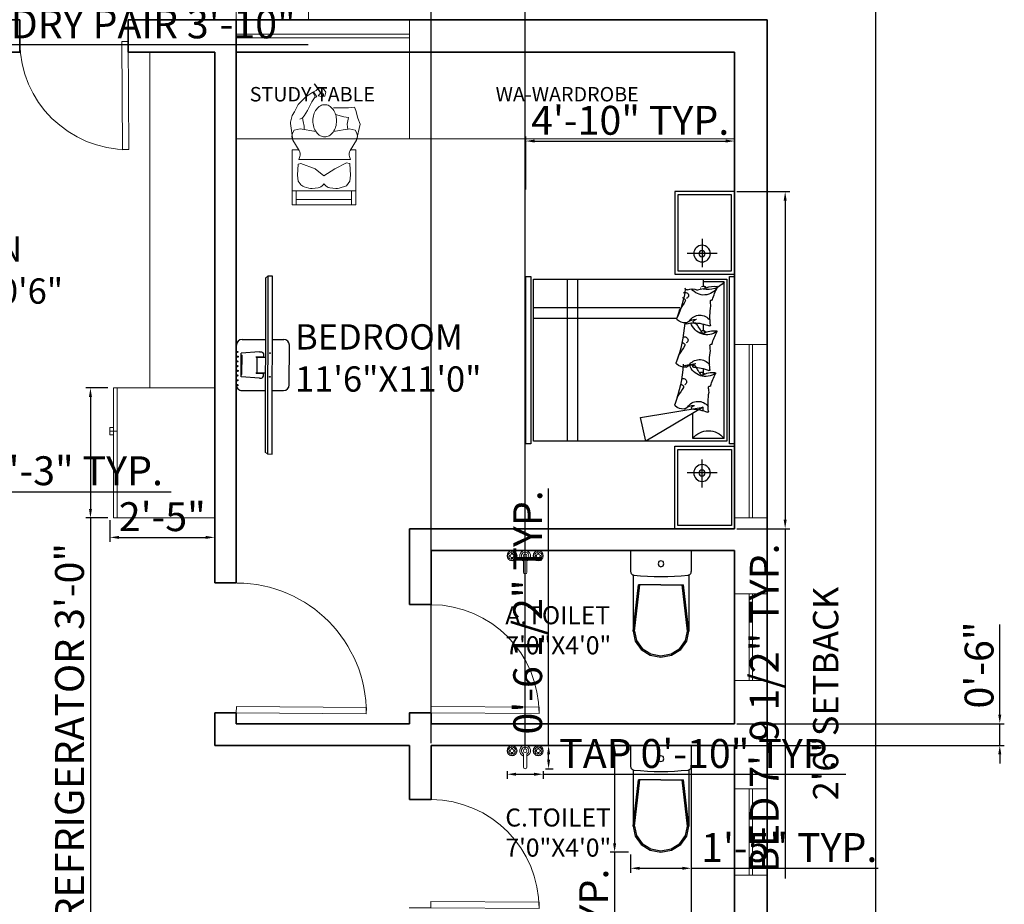
# Model space of a CAD drawing. Units: inches. Extents: x 3394 to 4794, y 965 to 1718.
# Tile 10 of 15: x 3704 to 3976, y 1338 to 1583. Entities that reach past the tile are written whole.
import ezdxf

# ---------------------------------------------------------------- set-up
doc = ezdxf.new("R2010")
doc.units = ezdxf.units.IN
for name, color, linetype, lineweight in [('A-ANNO-DIMS', 2, 'Continuous', 13), ('A-ANNO-TEXT', 7, 'Continuous', 18), ('A-AREA-IDEN', 7, 'Continuous', 18), ('A-DOOR', 4, 'Continuous', 18), ('A-EQPM', 8, 'Continuous', 18), ('A-FLOR-CASE', 8, 'Continuous', 18), ('A-FLOR-STRS', 7, 'Continuous', 18), ('A-GLAZ', 4, 'Continuous', 18), ('A-WALL', 7, 'Continuous', 35), ('C-PROP', 7, 'Continuous', 25), ('NOITHAT', 21, 'Continuous', 18), ('Сантехника', 7, 'Continuous', 18)]:
    doc.layers.add(name, color=color, linetype=linetype, lineweight=lineweight)
for name, color, linetype in [('FUR', 42, 'Continuous'), ('HA', 9, 'Continuous'), ('HID', 11, 'Continuous'), ('SAN', 5, 'Continuous'), ('SANTEH', 7, 'Continuous'), ('window', 130, 'Continuous')]:
    doc.layers.add(name, color=color, linetype=linetype)
doc.styles.get("Standard").update_dxf_attribs({"font": 'arial.ttf'})
doc.dimstyles.new('ISO-25', dxfattribs={"dimtxt": 8, "dimasz": 2.5, "dimexe": 1.25, "dimexo": 0.625, "dimtad": 1, "dimlunit": 3, "dimtxsty": 'Standard', "dimcen": 2.5, "dimadec": 0, "dimazin": 0, "dimtfac": 1, "dimtmove": 0, "dimatfit": 3, "dimfxl": 1, "dimarcsym": 0})

# ---------------------------------------------------------------- blocks, each defined once
blk = doc.blocks.new('Refrigerator-2 door - 36 in top')
for p, q in [((0, -26.999999), (36, -26.999999)), ((12, -26.999999), (12, -28.999999)), ((11, -27.999999), (11, -28.999999)), ((11, -28.999999), (13, -28.999999)), ((13, -28.999999), (13, -27.999999))]:
    blk.add_line(p, q)
blk.add_lwpolyline([(0, -27.999999), (0, 0), (36, 0), (36, -27.999999)], close=True)
blk = doc.blocks.new('Faucet - Bathroom top')
for p, q in [((-4.107, 0.125), (-4.375, 0.125)), ((-3.75, 0.4788), (-3.75, 0.75)), ((-3.5, 0.482), (-3.5, 0.75)), ((-3.1461, 0.125), (-2.875, 0.125)), ((3.143, 0.125), (2.875, 0.125)), ((3.5, 0.4788), (3.5, 0.75)), ((3.75, 0.482), (3.75, 0.75)), ((4.1039, 0.125), (4.375, 0.125)), ((-4.1039, -0.125), (-4.375, -0.125)), ((-3.75, -0.4821), (-3.75, -0.75)), ((-3.5, -0.4789), (-3.5, -0.75)), ((-3.143, -0.125), (-2.875, -0.125)), ((-0.5, -0.8639), (-0.5, -4.5)), ((0.5, -4.5), (0.5, -0.8631)), ((3.1461, -0.125), (2.875, -0.125)), ((3.5, -0.4821), (3.5, -0.75)), ((3.75, -0.4789), (3.75, -0.75)), ((4.107, -0.125), (4.375, -0.125))]:
    blk.add_line(p, q)
for centre, radius in [((-3.625, 0), 1.375), ((-4.625, 0), 0.2795), ((-3.625, 0), 0.5), ((-3.625, 1), 0.2795), ((-2.625, 0), 0.2795), ((0, 0), 0.5), ((3.625, 0), 1.375), ((2.625, 0), 0.2795), ((3.625, 0), 0.5), ((3.625, 1), 0.2795), ((4.625, 0), 0.2795), ((-3.625, -1), 0.2795), ((3.625, -1), 0.2795)]:
    blk.add_circle(centre, radius)
for centre, radius, start, end in [((-3.625, 0), 1, 105.2407, 164.2093), ((-3.625, 0), 1, 16.44125, 74.07887), ((0, 0), 1.5, 289.6514, 250.3603), ((0, 0), 1, 300.3431, 239.7554), ((3.625, 0), 1, 106.12, 164.0884), ((3.625, 0), 1, 16.23422, 73.90469), ((-3.625, 0), 1, 196.2342, 253.9047), ((-3.625, 0), 1, 286.12, 344.0884), ((3.625, 0), 1, 196.4413, 254.0789), ((3.625, 0), 1, 285.2407, 344.2093), ((0, -4.5), 0.5, 180, 0)]:
    blk.add_arc(centre, radius, start, end)
blk = doc.blocks.new('*U5')
for p, q in [((0, 0), (0, -6)), ((30, 0), (30, -6))]:
    blk.add_line(p, q)
blk.add_lwpolyline([(0, 0), (0, 30), (1.75, 30), (1.75, 0)], close=True)
blk.add_arc((0, 0), 30, 0, 90)
blk = doc.blocks.new('WC 2 Symb_109')
at = {"layer": 'SANTEH'}
for p, q in [((0, 0), (0, 380)), ((0, 380), (132.4, 380)), ((153.6, 364.9), (506.8, 364.9)), ((506.3, 364.9), (215.7, 330.9)), ((506.3, 356), (215.7, 322)), ((215.7, 190), (215.7, 330.9)), ((215.7, 190), (215.7, 49.1)), ((153.8, 15.1), (506.8, 15.1)), ((506.3, 24), (215.7, 58)), ((506.3, 15.1), (215.7, 49.1)), ((0, 0), (132.4, 0))]:
    blk.add_line(p, q, dxfattribs=at)
for points in [[(154.6, 360.1), (153.9, 364.1), (152.3, 367.9), (150.2, 371.3), (147.4, 374.3), (144.1, 376.7), (140.5, 378.5), (136.5, 379.6), (132.4, 380)], [(154.6, 19.7), (158.6, 62.1), (161.4, 104.7), (163.1, 147.3), (163.7, 189.9), (163.1, 232.5), (161.4, 275.1), (158.6, 317.7), (154.6, 360.1)], [(506.3, 24), (565.5, 36.6), (615.7, 72.6), (649.2, 126.5), (661, 190), (649.2, 253.5), (615.7, 307.4), (565.5, 343.4), (506.3, 356)], [(506.8, 15.1), (569.2, 28.4), (622.2, 66.3), (657.6, 123.1), (670, 190), (657.6, 256.9), (622.2, 313.7), (569.2, 351.6), (506.8, 364.9)], [(132.4, 0), (136.5, 0.4), (140.4, 1.5), (144.1, 3.2), (147.3, 5.6), (150.1, 8.6), (152.3, 12), (153.8, 15.7), (154.6, 19.7)]]:
    blk.add_lwpolyline(points, dxfattribs=at)
blk.add_lwpolyline([(83.6, 208.5), (70.4, 203.1), (64.9, 190), (70.4, 176.9), (83.6, 171.5), (96.8, 176.9), (102.2, 190), (96.8, 203.1)], close=True, dxfattribs=at)
blk = doc.blocks.new('*U11')
for p, q in [((0, 0), (0, -6)), ((36, 0), (36, -6))]:
    blk.add_line(p, q)
blk.add_lwpolyline([(0, 0), (0, 36), (1.75, 36), (1.75, 0)], close=True)
blk.add_arc((0, 0), 36, 0, 90)
blk = doc.blocks.new('A$C73A16738')
at = {"layer": 'FUR'}
for p, q in [((1.15, 2.3893), (1.1, 2.1643)), ((1.7, 2.0643), (1.15, 2.3893)), ((1.6, 2.3643), (1.6, 2.1234)), ((1.9, 2.3643), (1.6, 2.3643)), ((1.9, 2.3643), (1.9, 0.8643)), ((1.1, 2.1643), (1.7, 2.0643)), ((1.7, 2.099), (1.7, 2.0643)), ((1.7, 1.6955), (1.7, 1.7349)), ((1.7, 1.2682), (1.7, 1.3299)), ((1.7, 0.8393), (1.7, 0.9036)), ((1.9, 0.8643), (1.7, 0.8643))]:
    blk.add_line(p, q, dxfattribs=at)
for points in [[(1.428, 2.4393), (2, 2.4393), (2, 3.2287), (1.428, 3.2287)], [(1.458, 2.4693), (1.97, 2.4693), (1.97, 3.1987), (1.458, 3.1987)], [(0, 2.4143), (0, 0.8143), (0.05, 0.8143), (0.05, 2.4143)], [(0.075, 0.8393), (1.925, 0.8393), (1.925, 2.3893), (0.075, 2.3893)], [(1.95, 2.4143), (1.95, 0.8143), (2, 0.8143), (2, 2.4143)], [(1.428, 0.7893), (2, 0.7893), (2, 0), (1.428, 0)], [(1.458, 0.7593), (1.97, 0.7593), (1.97, 0.03), (1.458, 0.03)]]:
    blk.add_lwpolyline(points, close=True, dxfattribs=at)
for centre, start, end in [((1.75, 2.4806), 217.78263, 322.21737), ((1.75, 0.7481), 37.78263, 105.27469)]:
    blk.add_arc(centre, 0.1898, start, end, dxfattribs=at)
at = {"layer": 'HA'}
for p, q in [((0.4, 2.3893), (0.4, 0.8393)), ((0.5, 2.3893), (0.5, 0.8393)), ((1.4456, 1.2143), (0.075, 1.2143)), ((1.4772, 1.1143), (0.075, 1.1143))]:
    blk.add_line(p, q, dxfattribs=at)
at = {"layer": 'HID'}
for centre, radius, start, end in [((1.5102, 1.9654), 0.1174, 87.33771, 131.66603), ((1.515, 2.0683), 0.0144, 51.60711, 87.33771), ((1.6169, 2.1969), 0.1496, 231.60711, 269.78448), ((1.5925, 2.0742), 0.0072, 92.73629, 208.29854), ((1.5692, 2.5605), 0.4796, 272.73629, 290.95899), ((1.7434, 2.1059), 0.0072, 352.72477, 110.95899), ((2.3483, 2.0286), 0.6026, 172.72477, 190.27016), ((1.4417, 2.0424), 0.0144, 131.66603, 199.44651), ((0.016, 1.539), 1.4976, 4.58522, 19.44651), ((0.016, 1.539), 1.4976, 16.38601, 19.44651), ((1.6496, 2.1284), 0.1197, 212.76276, 323.89219), ((1.628, 2.0933), 0.0475, 208.29854, 255.78909), ((1.4666, 1.9655), 0.0144, 196.38601, 223.79553), ((0.9264, 1.5508), 0.6667, 29.04896, 37.38232), ((2.0379, 1.8684), 0.2875, 169.41677, 179.30852), ((1.5097, 1.8233), 0.0319, 112.70152, 147.15561), ((1.5097, 1.8214), 0.0305, 232.35651, 65.77621), ((1.5029, 1.8394), 0.0144, 102.64257, 112.70152), ((1.4966, 1.8675), 0.0144, 282.64257, 29.04896), ((1.7576, 1.8718), 0.0072, 179.30852, 290.68903), ((1.7627, 1.8583), 0.0072, 16.21957, 110.68903), ((2.3483, 2.0286), 0.6026, 196.21957, 208.21138), ((1.7225, 1.6087), 0.1623, 53.89466, 162.39517), ((1.5829, 2.1606), 0.4796, 272.73629, 290.95899), ((2.8537, 0.9606), 1.4182, 145.83293, 150.02451), ((3.1426, 2.3695), 1.6108, 202.70178, 202.72062), ((1.6834, 1.7584), 0.0288, 232.66199, 339.15728), ((1.6862, 1.7531), 0.0072, 38.83153, 145.83293), ((1.788, 1.9236), 0.1919, 239.92106, 277.12402), ((0.088, 1.8308), 1.6108, 356.49824, 357.28883), ((1.7571, 1.706), 0.0072, 352.72477, 110.95899), ((2.362, 1.6287), 0.6026, 172.72477, 190.27016), ((1.8109, 1.7404), 0.0072, 277.12402, 28.21138), ((1.8109, 1.7404), 0.0072, 277.12402, 28.21138), ((1.4554, 1.6425), 0.0144, 131.66603, 199.44651), ((0.0297, 1.1391), 1.4976, 4.58522, 19.44651), ((0.0297, 1.1391), 1.4976, 16.38601, 19.44651), ((1.5239, 1.5655), 0.1174, 87.33771, 131.66603), ((1.5236, 1.6535), 0.0144, 67.16626, 184.34216), ((1.5745, 1.7743), 0.1167, 247.16626, 295.7613), ((1.5287, 1.6684), 0.0144, 51.60711, 87.33771), ((1.6306, 1.797), 0.1496, 231.60711, 269.78448), ((1.6633, 1.7284), 0.1197, 212.76276, 323.89219), ((1.6062, 1.6743), 0.0072, 92.73629, 208.29854), ((1.6417, 1.6934), 0.0475, 208.29854, 255.78909), ((1.4803, 1.5656), 0.0144, 196.38601, 223.79553), ((0.9401, 1.1509), 0.6667, 29.04896, 37.38232), ((2.0516, 1.4685), 0.2875, 169.41677, 179.30852), ((1.5234, 1.4234), 0.0319, 112.70152, 147.15561), ((1.5234, 1.4215), 0.0305, 232.35651, 65.77621), ((1.5166, 1.4395), 0.0144, 102.64257, 112.70152), ((1.5103, 1.4676), 0.0144, 282.64257, 29.04896), ((1.7713, 1.4719), 0.0072, 179.30852, 290.68903), ((1.7764, 1.4584), 0.0072, 16.21957, 110.68903), ((2.362, 1.6287), 0.6026, 196.21957, 208.21138), ((1.7362, 1.2088), 0.1623, 53.89466, 162.39517), ((2.8674, 0.5607), 1.4182, 145.83293, 150.02451), ((3.1563, 1.9695), 1.6108, 202.70178, 202.72062), ((1.6971, 1.3585), 0.0288, 232.66199, 339.15728), ((1.6999, 1.3531), 0.0072, 38.83153, 145.83293), ((1.8017, 1.5237), 0.1919, 239.92106, 277.12402), ((0.1017, 1.4309), 1.6108, 356.49824, 357.28883), ((1.8246, 1.3404), 0.0072, 277.12402, 28.21138), ((1.8246, 1.3404), 0.0072, 277.12402, 28.21138), ((1.4601, 1.2163), 0.0144, 131.66603, 199.44651), ((1.5286, 1.1394), 0.1174, 87.33771, 131.66603), ((1.5373, 1.2536), 0.0144, 67.16626, 184.34216), ((1.5334, 1.2423), 0.0144, 51.60711, 87.33771), ((1.6353, 1.3709), 0.1496, 231.60711, 269.78448), ((1.5882, 1.3744), 0.1167, 247.16626, 295.7613), ((1.6681, 1.3023), 0.1197, 212.76276, 323.89219), ((1.6109, 1.2482), 0.0072, 92.73629, 208.29854), ((1.6464, 1.2673), 0.0475, 208.29854, 255.78909), ((1.5877, 1.7344), 0.4796, 272.73629, 290.95899), ((1.7618, 1.2798), 0.0072, 352.72477, 110.95899), ((2.3667, 1.2026), 0.6026, 172.72477, 190.27016), ((0.6883, 0.8412), 0.8439, 6.22401, 26.03262), ((0.0344, 0.713), 1.4976, 16.38601, 19.44651), ((1.485, 1.1395), 0.0144, 196.38601, 223.79553), ((0.9449, 0.7248), 0.6667, 29.04896, 37.38232), ((1.5151, 1.0415), 0.0144, 282.64257, 29.04896), ((2.0564, 1.0424), 0.2875, 169.41677, 179.30852), ((1.7761, 1.0457), 0.0072, 179.30852, 290.68903), ((1.7812, 1.0323), 0.0072, 16.21957, 110.68903), ((1.5281, 0.9972), 0.0319, 112.70152, 147.15561), ((1.5282, 0.9954), 0.0305, 232.35651, 65.77621), ((1.5214, 1.0134), 0.0144, 102.64257, 112.70152), ((1.5929, 1.0482), 0.1167, 247.16626, 295.7613), ((1.7054, 0.84), 0.1504, 29.35981, 142.42811), ((1.5813, 0.5283), 0.4195, 73.75237, 81.4605), ((2.3667, 1.2026), 0.6026, 196.21957, 208.21138), ((1.5421, 0.9274), 0.0144, 67.16626, 184.34216), ((3.1611, 1.5434), 1.6108, 202.70178, 202.72062), ((1.7018, 0.9324), 0.0288, 232.66199, 339.15728), ((1.7047, 0.927), 0.0072, 38.83153, 145.83293), ((0.1065, 1.0048), 1.6108, 356.49824, 357.28883), ((1.8064, 1.0976), 0.1919, 246.10926, 277.12402), ((1.8293, 0.9143), 0.0072, 277.12402, 28.21138), ((1.8293, 0.9143), 0.0072, 277.12402, 28.21138)]:
    blk.add_arc(centre, radius, start, end, dxfattribs=at)
at = {"layer": 'SAN'}
for p, q in [((1.6885, 2.8351), (1.6885, 2.5658)), ((1.8316, 2.6947), (1.5465, 2.6947)), ((1.6885, 0.4536), (1.6885, 0.7229)), ((1.8316, 0.594), (1.5465, 0.594))]:
    blk.add_line(p, q, dxfattribs=at)
for centre, radius in [((1.6885, 2.6947), 0.08), ((1.6885, 2.6947), 0.03), ((1.6885, 0.594), 0.08), ((1.6885, 0.594), 0.03)]:
    blk.add_circle(centre, radius, dxfattribs=at)
blk = doc.blocks.new('TV')
at = {"color": 0}
for p, q in [((3967.27, 1784.85), (3967.05, 1784.65)), ((3967.76, 1763.68), (3967.54, 1763.86))]:
    blk.add_line(p, q, dxfattribs=at)
at = {"layer": 'window'}
for p, q in [((3967.54, 1763.86), (3967.05, 1784.65)), ((3964.41, 1777.23), (3967.22, 1777.3)), ((3968.01, 1777.32), (3969.36, 1777.35)), ((3966.53, 1775.82), (3964.33, 1775.61)), ((3964.34, 1775.34), (3964.45, 1775.34)), ((3964.34, 1775.31), (3964.43, 1775.32)), ((3966.14, 1775.2), (3967.01, 1775.22)), ((3966.14, 1775.18), (3967.27, 1775.2)), ((3966.14, 1775.18), (3966.14, 1775.2)), ((3966.3, 1773.29), (3966.26, 1775.18)), ((3964.39, 1773.06), (3964.48, 1773.06)), ((3964.39, 1773.04), (3964.5, 1773.04)), ((3966.19, 1773.28), (3967.31, 1773.31)), ((3966.19, 1773.26), (3967.05, 1773.28)), ((3966.19, 1773.26), (3966.19, 1773.28)), ((3966.61, 1772.66), (3964.4, 1772.77)), ((3964.55, 1771.15), (3967.36, 1771.22)), ((3968.15, 1771.24), (3969.5, 1771.27))]:
    blk.add_line(p, q, dxfattribs=at)
for points in [[(3968.33, 1763.69), (3967.83, 1784.86), (3967.27, 1784.85), (3967.76, 1763.68), (3968.33, 1763.69)], [(3963.86, 1771.81), (3963.75, 1776.54)], [(3970.16, 1771.96), (3970.05, 1776.69)], [(3964.4, 1772.77), (3964.33, 1775.61)], [(3964.48, 1773.06), (3964.43, 1775.32)], [(3964.5, 1773.04), (3964.45, 1775.34)]]:
    blk.add_lwpolyline(points, dxfattribs=at)
for points in [[(3966.53, 1775.82, -0.263666), (3966.93, 1775.69), (3967, 1775.57), (3967.01, 1775.22)], [(3966.61, 1772.66, 0.263666), (3967, 1772.81), (3967.06, 1772.93), (3967.05, 1773.28)]]:
    blk.add_lwpolyline(points, format="xyb", dxfattribs=at)
for centre, radius in [((3963.91, 1775.73), 0.0679), ((3963.93, 1775.17), 0.0679), ((3967.77, 1775.68), 0.0451), ((3963.94, 1774.6), 0.0679), ((3963.95, 1774.04), 0.0679), ((3963.97, 1773.48), 0.0679), ((3963.98, 1772.92), 0.0679), ((3967.83, 1772.86), 0.0451), ((3963.99, 1772.35), 0.0679), ((3964.01, 1771.79), 0.0679)]:
    blk.add_circle(centre, radius, dxfattribs=at)
for centre, start, end in [((3964.42, 1776.56), 91.3414, 181.3414), ((3969.38, 1776.67), 1.3414, 91.3414), ((3964.53, 1771.83), 181.3414, 271.3414), ((3969.49, 1771.94), 271.3414, 1.3414)]:
    blk.add_arc(centre, 0.676, start, end, dxfattribs=at)
blk = doc.blocks.new('WIN-48IN')
for p, q in [((9, 48), (0, 48)), ((4, 0), (4, 48)), ((5, 0), (5, 48)), ((9, 0), (0, 0))]:
    blk.add_line(p, q)
blk = doc.blocks.new('WIN-24IN')
for p, q in [((0, 9), (0, 0)), ((24, 9), (24, 0)), ((0, 5), (24, 5)), ((0, 4), (24, 4))]:
    blk.add_line(p, q)
blk = doc.blocks.new('*D78')
at = {"layer": 'A-ANNO-DIMS', "color": 0, "lineweight": -2, "transparency": 16777216}
for p, q in [((3838.73, 1374.56), (3838.73, 1372.43)), ((3848.73, 1374.56), (3848.73, 1372.43)), ((3841.23, 1373.68), (3846.23, 1373.68)), ((3848.73, 1373.68), (3932.51, 1373.68))]:
    blk.add_line(p, q, dxfattribs=at)
at = {"layer": 'A-ANNO-DIMS', "color": 0, "transparency": 16777216}
for points in [[(3841.23, 1374.1), (3841.23, 1373.27), (3838.73, 1373.68)], [(3846.23, 1374.1), (3846.23, 1373.27), (3848.73, 1373.68)]]:
    blk.add_solid(points, dxfattribs=at)
at = {"layer": 'Defpoints', "color": 0, "transparency": 16777216}
for p in [(3838.73, 1375.18), (3848.73, 1375.18), (3848.73, 1373.68)]:
    blk.add_point(p, dxfattribs=at)
at = {"layer": 'A-ANNO-DIMS', "color": 0, "transparency": 16777216, "insert": (3891.87, 1378.39), "char_height": 8, "attachment_point": 5}
blk.add_mtext('TAP 0\'-10" TYP.', dxfattribs=at)
blk = doc.blocks.new('*D79')
at = {"layer": 'A-ANNO-DIMS', "color": 0, "lineweight": -2, "transparency": 16777216}
for p, q in [((3850.23, 1381.68), (3850.23, 1452.84)), ((3849.36, 1381.68), (3851.48, 1381.68)), ((3850.23, 1377.68), (3850.23, 1379.18)), ((3849.36, 1375.18), (3851.48, 1375.18))]:
    blk.add_line(p, q, dxfattribs=at)
at = {"layer": 'A-ANNO-DIMS', "color": 0, "transparency": 16777216}
for points in [[(3849.82, 1379.18), (3850.65, 1379.18), (3850.23, 1381.68)], [(3849.82, 1377.68), (3850.65, 1377.68), (3850.23, 1375.18)]]:
    blk.add_solid(points, dxfattribs=at)
at = {"layer": 'Defpoints', "color": 0, "transparency": 16777216}
for p in [(3848.73, 1381.68), (3850.23, 1381.68), (3848.73, 1375.18)]:
    blk.add_point(p, dxfattribs=at)
at = {"layer": 'A-ANNO-DIMS', "color": 0, "transparency": 16777216, "insert": (3845.47, 1418.51), "char_height": 8, "attachment_point": 5, "rotation": 90}
blk.add_mtext('0\'-6 1/2" TYP.', dxfattribs=at)
blk = doc.blocks.new('*D80')
at = {"layer": 'A-ANNO-DIMS', "color": 0, "lineweight": -2, "transparency": 16777216}
for p, q in [((3872.33, 1381.68), (3867.26, 1381.68)), ((3868.51, 1379.18), (3868.51, 1354.58)), ((3872.33, 1352.08), (3867.26, 1352.08)), ((3868.51, 1352.08), (3868.51, 1258.87))]:
    blk.add_line(p, q, dxfattribs=at)
at = {"layer": 'A-ANNO-DIMS', "color": 0, "transparency": 16777216}
for points in [[(3868.09, 1379.18), (3868.93, 1379.18), (3868.51, 1381.68)], [(3868.09, 1354.58), (3868.93, 1354.58), (3868.51, 1352.08)]]:
    blk.add_solid(points, dxfattribs=at)
at = {"layer": 'Defpoints', "color": 0, "transparency": 16777216}
for p in [(3872.95, 1381.68), (3868.51, 1352.08), (3872.95, 1352.08)]:
    blk.add_point(p, dxfattribs=at)
at = {"layer": 'A-ANNO-DIMS', "color": 0, "transparency": 16777216, "insert": (3863.75, 1304.22), "char_height": 8, "attachment_point": 5, "rotation": 90}
blk.add_mtext('WC 2\'-5 1/2" TYP.', dxfattribs=at)
blk = doc.blocks.new('*D81')
at = {"layer": 'A-ANNO-DIMS', "color": 0, "lineweight": -2, "transparency": 16777216}
for p, q in [((3872.95, 1351.45), (3872.95, 1346.38)), ((3889.74, 1351.45), (3889.74, 1346.38)), ((3875.45, 1347.63), (3887.24, 1347.63)), ((3889.74, 1347.63), (3941.51, 1347.63))]:
    blk.add_line(p, q, dxfattribs=at)
at = {"layer": 'A-ANNO-DIMS', "color": 0, "transparency": 16777216}
for points in [[(3875.45, 1348.05), (3875.45, 1347.22), (3872.95, 1347.63)], [(3887.24, 1348.05), (3887.24, 1347.22), (3889.74, 1347.63)]]:
    blk.add_solid(points, dxfattribs=at)
at = {"layer": 'Defpoints', "color": 0, "transparency": 16777216}
for p in [(3872.95, 1352.08), (3889.74, 1352.08), (3889.74, 1347.63)]:
    blk.add_point(p, dxfattribs=at)
at = {"layer": 'A-ANNO-DIMS', "color": 0, "transparency": 16777216, "insert": (3916.88, 1352.34), "char_height": 8, "attachment_point": 5}
blk.add_mtext('1\'-5" TYP.', dxfattribs=at)
blk = doc.blocks.new('*D86')
at = {"layer": 'A-ANNO-DIMS', "color": 0, "lineweight": -2, "transparency": 16777216}
for p, q in [((3902.37, 1535.06), (3917, 1535.06)), ((3915.75, 1532.56), (3915.75, 1444.18)), ((3902.37, 1441.68), (3917, 1441.68)), ((3915.75, 1441.68), (3915.75, 1344.8))]:
    blk.add_line(p, q, dxfattribs=at)
at = {"layer": 'A-ANNO-DIMS', "color": 0, "transparency": 16777216}
for points in [[(3915.34, 1532.56), (3916.17, 1532.56), (3915.75, 1535.06)], [(3915.34, 1444.18), (3916.17, 1444.18), (3915.75, 1441.68)]]:
    blk.add_solid(points, dxfattribs=at)
at = {"layer": 'Defpoints', "color": 0, "transparency": 16777216}
for p in [(3901.74, 1535.06), (3901.74, 1441.68), (3915.75, 1441.68)]:
    blk.add_point(p, dxfattribs=at)
at = {"layer": 'A-ANNO-DIMS', "color": 0, "transparency": 16777216, "insert": (3910.99, 1391.99), "char_height": 8, "attachment_point": 5, "rotation": 90}
blk.add_mtext('BED 7\'-9 1/2" TYP.', dxfattribs=at)
blk = doc.blocks.new('*D87')
at = {"layer": 'A-ANNO-DIMS', "color": 0, "lineweight": -2, "transparency": 16777216}
for p, q in [((3843.9, 1535.69), (3843.9, 1550.32)), ((3846.4, 1549.07), (3899.24, 1549.07)), ((3901.74, 1535.69), (3901.74, 1550.32))]:
    blk.add_line(p, q, dxfattribs=at)
at = {"layer": 'A-ANNO-DIMS', "color": 0, "transparency": 16777216}
for points in [[(3846.4, 1549.49), (3846.4, 1548.65), (3843.9, 1549.07)], [(3899.24, 1549.49), (3899.24, 1548.65), (3901.74, 1549.07)]]:
    blk.add_solid(points, dxfattribs=at)
at = {"layer": 'Defpoints', "color": 0, "transparency": 16777216}
for p in [(3901.74, 1549.07), (3843.9, 1535.06), (3901.74, 1535.06)]:
    blk.add_point(p, dxfattribs=at)
at = {"layer": 'A-ANNO-DIMS', "color": 0, "transparency": 16777216, "insert": (3872.82, 1553.78), "char_height": 8, "attachment_point": 5}
blk.add_mtext('4\'-10" TYP.', dxfattribs=at)
blk = doc.blocks.new('*D88')
at = {"layer": 'A-ANNO-DIMS', "color": 0, "lineweight": -2, "transparency": 16777216}
for p, q in [((3637.38, 1453.56), (3637.38, 1450.71)), ((3652.23, 1453.56), (3652.23, 1450.7)), ((3639.88, 1451.96), (3649.73, 1451.96)), ((3652.23, 1451.95), (3745.7, 1451.93))]:
    blk.add_line(p, q, dxfattribs=at)
at = {"layer": 'A-ANNO-DIMS', "color": 0, "transparency": 16777216}
for points in [[(3639.88, 1452.37), (3639.88, 1451.54), (3637.38, 1451.96)], [(3649.73, 1452.37), (3649.73, 1451.54), (3652.23, 1451.95)]]:
    blk.add_solid(points, dxfattribs=at)
at = {"layer": 'Defpoints', "color": 0, "transparency": 16777216}
for p in [(3637.38, 1454.19), (3652.23, 1454.18), (3652.23, 1451.95)]:
    blk.add_point(p, dxfattribs=at)
at = {"layer": 'A-ANNO-DIMS', "color": 0, "transparency": 16777216, "insert": (3700.21, 1456.71), "char_height": 8, "attachment_point": 5, "rotation": 359.9851}
blk.add_mtext('STOOL 1\'-3" TYP.', dxfattribs=at)
blk = doc.blocks.new('*D90')
at = {"layer": 'A-ANNO-DIMS', "color": 0, "lineweight": -2, "transparency": 16777216}
for p, q in [((3728.12, 1480.68), (3722.09, 1480.68)), ((3723.34, 1478.18), (3723.34, 1447.18)), ((3728.12, 1444.68), (3722.09, 1444.68)), ((3723.34, 1444.68), (3723.34, 1328.18))]:
    blk.add_line(p, q, dxfattribs=at)
at = {"layer": 'A-ANNO-DIMS', "color": 0, "transparency": 16777216}
for points in [[(3722.93, 1478.18), (3723.76, 1478.18), (3723.34, 1480.68)], [(3722.93, 1447.18), (3723.76, 1447.18), (3723.34, 1444.68)]]:
    blk.add_solid(points, dxfattribs=at)
at = {"layer": 'Defpoints', "color": 0, "transparency": 16777216}
for p in [(3728.74, 1480.68), (3723.34, 1444.68), (3728.74, 1444.68)]:
    blk.add_point(p, dxfattribs=at)
at = {"layer": 'A-ANNO-DIMS', "color": 0, "transparency": 16777216, "insert": (3718.58, 1385.18), "char_height": 8, "attachment_point": 5, "rotation": 90}
blk.add_mtext('REFRIGERATOR 3\'-0"', dxfattribs=at)
blk = doc.blocks.new('*D91')
at = {"layer": 'A-ANNO-DIMS', "color": 0, "lineweight": -2, "transparency": 16777216}
for p, q in [((3728.74, 1444.06), (3728.74, 1438.03)), ((3757.74, 1444.06), (3757.74, 1438.03)), ((3731.24, 1439.28), (3755.24, 1439.28))]:
    blk.add_line(p, q, dxfattribs=at)
at = {"layer": 'A-ANNO-DIMS', "color": 0, "transparency": 16777216}
for points in [[(3731.24, 1439.7), (3731.24, 1438.87), (3728.74, 1439.28)], [(3755.24, 1439.7), (3755.24, 1438.87), (3757.74, 1439.28)]]:
    blk.add_solid(points, dxfattribs=at)
at = {"layer": 'Defpoints', "color": 0, "transparency": 16777216}
for p in [(3728.74, 1444.68), (3757.74, 1444.68), (3757.74, 1439.28)]:
    blk.add_point(p, dxfattribs=at)
at = {"layer": 'A-ANNO-DIMS', "color": 0, "transparency": 16777216, "insert": (3743.24, 1443.99), "char_height": 8, "attachment_point": 5}
blk.add_mtext('2\'-5"', dxfattribs=at)
blk = doc.blocks.new('*D92')
at = {"layer": 'A-ANNO-DIMS', "color": 0, "lineweight": -2, "transparency": 16777216}
for p, q in [((3620.92, 1582.06), (3620.92, 1574.52)), ((3667.02, 1582.06), (3667.02, 1574.52)), ((3623.42, 1575.77), (3664.52, 1575.77)), ((3667.02, 1575.77), (3783.6, 1575.77))]:
    blk.add_line(p, q, dxfattribs=at)
at = {"layer": 'A-ANNO-DIMS', "color": 0, "transparency": 16777216}
for points in [[(3623.42, 1576.18), (3623.42, 1575.35), (3620.92, 1575.77)], [(3664.52, 1576.18), (3664.52, 1575.35), (3667.02, 1575.77)]]:
    blk.add_solid(points, dxfattribs=at)
at = {"layer": 'Defpoints', "color": 0, "transparency": 16777216}
for p in [(3620.92, 1582.68), (3667.02, 1582.68), (3667.02, 1575.77)]:
    blk.add_point(p, dxfattribs=at)
at = {"layer": 'A-ANNO-DIMS', "color": 0, "transparency": 16777216, "insert": (3726.56, 1580.48), "char_height": 8, "attachment_point": 5}
blk.add_mtext('LAUNDRY PAIR 3\'-10"', dxfattribs=at)
blk = doc.blocks.new('*D125')
at = {"layer": 'A-ANNO-DIMS', "color": 0, "lineweight": -2, "transparency": 16777216}
for p, q in [((3889.74, 1381.06), (3889.74, 987.36)), ((3901.74, 1381.06), (3901.74, 987.36)), ((3892.24, 988.61), (3899.24, 988.61)), ((3901.74, 988.61), (3926.01, 988.61))]:
    blk.add_line(p, q, dxfattribs=at)
at = {"layer": 'A-ANNO-DIMS', "color": 0, "transparency": 16777216}
for points in [[(3892.24, 989.03), (3892.24, 988.2), (3889.74, 988.61)], [(3899.24, 989.03), (3899.24, 988.2), (3901.74, 988.61)]]:
    blk.add_solid(points, dxfattribs=at)
at = {"layer": 'Defpoints', "color": 0, "transparency": 16777216}
for p in [(3889.74, 1381.68), (3901.74, 1381.68), (3901.74, 988.61)]:
    blk.add_point(p, dxfattribs=at)
at = {"layer": 'A-ANNO-DIMS', "color": 0, "transparency": 16777216, "insert": (3915.13, 993.32), "char_height": 8, "attachment_point": 5}
blk.add_mtext('1\'-0"', dxfattribs=at)
blk = doc.blocks.new('*D126')
at = {"layer": 'A-ANNO-DIMS', "color": 0, "lineweight": -2, "transparency": 16777216}
for p, q in [((3817.74, 1382.31), (3817.74, 1702.38)), ((3843.73, 1380.81), (3843.73, 1702.38)), ((3820.24, 1701.13), (3841.23, 1701.13))]:
    blk.add_line(p, q, dxfattribs=at)
at = {"layer": 'A-ANNO-DIMS', "color": 0, "transparency": 16777216}
for points in [[(3820.24, 1701.55), (3820.24, 1700.72), (3817.74, 1701.13)], [(3841.23, 1701.55), (3841.23, 1700.72), (3843.73, 1701.13)]]:
    blk.add_solid(points, dxfattribs=at)
at = {"layer": 'Defpoints', "color": 0, "transparency": 16777216}
for p in [(3843.73, 1701.13), (3817.74, 1381.68), (3843.73, 1380.18)]:
    blk.add_point(p, dxfattribs=at)
at = {"layer": 'A-ANNO-DIMS', "color": 0, "transparency": 16777216, "insert": (3830.74, 1705.77), "char_height": 8, "attachment_point": 5}
blk.add_mtext('2\'-2"', dxfattribs=at)
blk = doc.blocks.new('*D129')
at = {"layer": 'A-ANNO-DIMS', "color": 0, "lineweight": -2, "transparency": 16777216}
for p, q in [((3975.19, 1390.18), (3975.19, 1415.2)), ((3902.37, 1387.68), (3976.44, 1387.68)), ((3975.19, 1381.68), (3975.19, 1387.68)), ((3902.37, 1381.68), (3976.44, 1381.68)), ((3975.19, 1379.18), (3975.19, 1376.68))]:
    blk.add_line(p, q, dxfattribs=at)
at = {"layer": 'A-ANNO-DIMS', "color": 0, "transparency": 16777216}
for points in [[(3974.78, 1390.18), (3975.61, 1390.18), (3975.19, 1387.68)], [(3974.78, 1379.18), (3975.61, 1379.18), (3975.19, 1381.68)]]:
    blk.add_solid(points, dxfattribs=at)
at = {"layer": 'Defpoints', "color": 0, "transparency": 16777216}
for p in [(3901.74, 1387.68), (3975.19, 1387.68), (3901.74, 1381.68)]:
    blk.add_point(p, dxfattribs=at)
at = {"layer": 'A-ANNO-DIMS', "color": 0, "transparency": 16777216, "insert": (3970.49, 1403.94), "char_height": 8, "attachment_point": 5, "rotation": 90}
blk.add_mtext('0\'-6"', dxfattribs=at)

msp = doc.modelspace()

# ---------------------------------------------------------------- linework, layer by layer
at = {"layer": 'A-FLOR-CASE'}
for p, q in [((3811.745, 1582.682), (3811.745, 1549.682)), ((3739.745, 1573.682), (3739.745, 1480.682)), ((3763.745, 1549.682), (3901.745, 1549.682)), ((3739.745, 1480.682), (3757.745, 1480.682))]:
    msp.add_line(p, q, dxfattribs=at)
at = {"layer": 'A-FLOR-STRS'}
for p, q in [((3763.745, 1582.682), (3763.745, 1636.682)), ((3773.745, 1582.682), (3773.745, 1636.682)), ((3783.745, 1582.682), (3783.745, 1636.682))]:
    msp.add_line(p, q, dxfattribs=at)
at = {"layer": 'A-GLAZ'}
for p, q in [((3763.745, 1578.682), (3811.745, 1578.682)), ((3763.745, 1577.682), (3811.745, 1577.682))]:
    msp.add_line(p, q, dxfattribs=at)
at = {"layer": 'A-WALL'}
for p, q in [((3604.745, 1582.682), (3703.745, 1582.682)), ((3703.745, 1582.682), (3703.745, 1573.682)), ((3733.745, 1582.682), (3733.745, 1573.682)), ((3733.745, 1582.682), (3910.745, 1582.682)), ((3763.745, 1582.682), (3763.745, 1426.682)), ((3910.745, 1582.682), (3910.745, 1198.682)), ((3613.745, 1573.682), (3703.745, 1573.682)), ((3733.745, 1573.682), (3757.745, 1573.682)), ((3757.745, 1573.682), (3757.745, 1426.682)), ((3763.745, 1573.682), (3901.745, 1573.682)), ((3901.745, 1573.682), (3901.745, 1441.682)), ((3811.745, 1441.682), (3811.745, 1420.682)), ((3811.745, 1441.682), (3901.745, 1441.682)), ((3817.745, 1435.682), (3817.745, 1420.682)), ((3817.745, 1435.682), (3901.745, 1435.682)), ((3901.745, 1435.682), (3901.745, 1387.682)), ((3757.745, 1426.682), (3763.745, 1426.682)), ((3811.745, 1420.682), (3817.745, 1420.682)), ((3757.745, 1390.682), (3763.745, 1390.682)), ((3757.745, 1390.682), (3757.745, 1381.682)), ((3763.745, 1390.682), (3763.745, 1387.682)), ((3811.745, 1390.682), (3817.745, 1390.682)), ((3811.745, 1390.682), (3811.745, 1387.682)), ((3817.745, 1390.682), (3817.745, 1387.682)), ((3763.745, 1387.682), (3811.745, 1387.682)), ((3817.745, 1387.682), (3901.745, 1387.682)), ((3757.745, 1381.682), (3811.745, 1381.682)), ((3811.745, 1381.682), (3811.745, 1366.682)), ((3817.745, 1381.682), (3817.745, 1366.682)), ((3817.745, 1381.682), (3901.745, 1381.682)), ((3901.745, 1381.682), (3901.745, 1333.682)), ((3811.745, 1366.682), (3817.745, 1366.682))]:
    msp.add_line(p, q, dxfattribs=at)
at = {"layer": 'C-PROP'}
msp.add_line((3940.745, 1666.682), (3940.745, 1057.682), dxfattribs=at)
at = {"layer": 'NOITHAT'}
for p, q in [((3782.991, 1561.355), (3784.912, 1562.612)), ((3784.912, 1562.612), (3785.611, 1561.32)), ((3785.017, 1562.367), (3785.157, 1562.717)), ((3785.157, 1562.717), (3786.03, 1561.354)), ((3780.895, 1559.155), (3782.991, 1561.355)), ((3784.633, 1559.888), (3783.48, 1557.513)), ((3785.611, 1561.32), (3784.633, 1559.888)), ((3786.03, 1561.354), (3785.541, 1561.145)), ((3779.882, 1557.129), (3780.895, 1559.155)), ((3783.48, 1557.513), (3782.502, 1556.081)), ((3782.048, 1555.452), (3781.315, 1555.138)), ((3782.502, 1556.081), (3782.048, 1555.452)), ((3779.425, 1549.325), (3778.735, 1553.899)), ((3779.39, 1551.411), (3779.746, 1552.051)), ((3779.746, 1552.051), (3781.44, 1552.427)), ((3781.44, 1552.427), (3785.767, 1551.675)), ((3794.988, 1552.427), (3790.66, 1551.675)), ((3796.681, 1552.051), (3794.988, 1552.427)), ((3797.037, 1551.411), (3796.681, 1552.051)), ((3781.134, 1546.479), (3779.425, 1549.325)), ((3795.293, 1546.479), (3797.002, 1549.325)), ((3779.182, 1546.597), (3779.182, 1531.363)), ((3781.063, 1546.597), (3779.182, 1546.597)), ((3796.869, 1546.597), (3795.364, 1546.597)), ((3796.869, 1531.363), (3796.869, 1546.597)), ((3781.063, 1543.964), (3781.324, 1544.746)), ((3795.364, 1543.964), (3781.063, 1543.964)), ((3781.063, 1543.964), (3795.364, 1543.964)), ((3795.364, 1543.964), (3795.103, 1544.746)), ((3780.862, 1542.62), (3780.687, 1539.638)), ((3780.928, 1542.695), (3781.628, 1542.835)), ((3781.628, 1542.835), (3785.579, 1541.331)), ((3785.579, 1541.331), (3788.025, 1539.45)), ((3788.025, 1539.45), (3791.036, 1541.331)), ((3791.036, 1541.331), (3794.235, 1543.023)), ((3794.235, 1543.023), (3795.114, 1542.848)), ((3795.18, 1542.772), (3795.364, 1539.638)), ((3780.687, 1539.638), (3780.875, 1537.945)), ((3795.364, 1539.638), (3795.176, 1537.945)), ((3779.182, 1535.312), (3796.869, 1535.312)), ((3780.335, 1535.312), (3780.335, 1531.363)), ((3780.875, 1537.945), (3781.406, 1537.202)), ((3782.489, 1536.422), (3783.835, 1536.008)), ((3784.706, 1535.932), (3786.433, 1536.148)), ((3787.802, 1536.913), (3788.025, 1537.193)), ((3788.249, 1536.913), (3788.025, 1537.193)), ((3791.345, 1535.932), (3789.618, 1536.148)), ((3794.235, 1536.629), (3792.216, 1536.008)), ((3795.176, 1537.945), (3794.235, 1536.629)), ((3795.658, 1535.312), (3795.658, 1531.363)), ((3780.335, 1532.867), (3795.658, 1532.867)), ((3779.182, 1531.363), (3796.869, 1531.363))]:
    msp.add_line(p, q, dxfattribs=at)
at = {"layer": 'NOITHAT', "const_width": 0.409}
msp.add_lwpolyline([(3787.843, 1561.389), (3785.348, 1564.959)], dxfattribs=at)
at = {"layer": 'NOITHAT'}
for points in [[(3785.157, 1562.717), (3785.814, 1563.058), (3786.574, 1563.734), (3787.758, 1563.628), (3788.561, 1562.572), (3788.244, 1561.473), (3787.885, 1561.494), (3787.885, 1562.107), (3786.913, 1562.128), (3786.448, 1561.579), (3787.695, 1561.325)], [(3779.882, 1557.129), (3779.198, 1556.103), (3778.89, 1555.076), (3778.735, 1554.254), (3778.735, 1553.792)], [(3797.002, 1549.325), (3797.998, 1553.743), (3797.434, 1555.436), (3796.869, 1557.505), (3796.493, 1558.445), (3794.8, 1558.257), (3793.106, 1558.257), (3790.66, 1558.257)], [(3782.048, 1555.452), (3782.28, 1554.46), (3782.537, 1553.176), (3782.537, 1552.252)], [(3791.224, 1556.376), (3793.482, 1555.812), (3794.8, 1555.624), (3794.423, 1553.743), (3794.611, 1552.239)]]:
    msp.add_lwpolyline(points, dxfattribs=at)
msp.add_lwpolyline([(3784.946, 1554.682, 0.0740504), (3785.208, 1552.921, 0.0848007), (3785.906, 1551.528, 0.1063356), (3787.026, 1550.536, 0.1289555), (3788.226, 1550.222, 0.1289555), (3789.425, 1550.536, 0.1063356), (3790.545, 1551.528, 0.0848007), (3791.243, 1552.921, 0.0740504), (3791.506, 1554.682, 0.0740504), (3791.243, 1556.444, 0.0848007), (3790.545, 1557.836, 0.1063356), (3789.425, 1558.828, 0.1289555), (3788.226, 1559.143, 0.1289555), (3787.026, 1558.828, 0.1063356), (3785.906, 1557.836, 0.0848007), (3785.208, 1556.444, 0.0740504)], format="xyb", close=True, dxfattribs=at)
for centre, radius, start, end in [((3781.212, 1550.398), 2.084, 150.9331, 210.97654), ((3795.215, 1550.398), 2.084, 329.02346, 29.0669), ((3779.347, 1545.406), 2.084, 341.55636, 30.97654), ((3797.08, 1545.406), 2.084, 149.02346, 198.44364), ((3780.944, 1542.615), 0.0819, 101.30436, 176.63184), ((3795.098, 1542.767), 0.0819, 3.36816, 78.69563), ((3795.098, 1542.767), 0.0819, 3.36816, 78.69563), ((3783.102, 1538.414), 2.084, 215.55138, 252.90541), ((3784.447, 1538), 2.084, 252.90541, 277.12145), ((3786.174, 1538.216), 2.084, 277.12145, 321.32606), ((3789.876, 1538.216), 2.084, 218.67394, 262.87855), ((3791.604, 1538), 2.084, 262.87855, 287.09459)]:
    msp.add_arc(centre, radius, start, end, dxfattribs=at)

# ---------------------------------------------------------------- block references
at = {"layer": 'A-DOOR', "rotation": 180.3213350750104}
msp.add_blockref('*U5', (3733.778, 1576.682), dxfattribs=at)
at = {"layer": 'A-DOOR', "xscale": -1}
for name, p, rotation in [('*U11', (3763.745, 1390.649), 269.6786649249896), ('*U5', (3817.576, 1390.649), 269.6786649249897), ('*U5', (3817.576, 1336.649), 269.6786649249897)]:
    msp.add_blockref(name, p, dxfattribs=dict(at, rotation=rotation))
at = {"layer": 'A-EQPM', "xscale": 2.327319231123021, "yscale": 2.327319231123021, "zscale": 2.327319231123021, "rotation": 358.5430845181613}
msp.add_blockref('TV', (-5563.285, -2406.142), dxfattribs=at)
at = {"layer": 'A-EQPM', "rotation": 270}
msp.add_blockref('Refrigerator-2 door - 36 in top', (3757.745, 1480.682), dxfattribs=at)
at = {"layer": 'A-GLAZ'}
msp.add_blockref('WIN-48IN', (3901.745, 1444.682), dxfattribs=at)
for p, rotation in [((3901.744, 1423.682), 269.999999999998), ((3910.745, 1345.683), 90.00000000000524)]:
    msp.add_blockref('WIN-24IN', p, dxfattribs=dict(at, rotation=rotation))
at = {"layer": 'NOITHAT', "xscale": -28.92215291203286, "yscale": 28.92215291203286, "zscale": 28.92215291203286, "rotation": 180}
msp.add_blockref('A$C73A16738', (3843.9, 1535.063), dxfattribs=at)
at = {"layer": 'Сантехника'}
for p in [(3843.735, 1434.182), (3843.735, 1380.182)]:
    msp.add_blockref('Faucet - Bathroom top', p, dxfattribs=at)
at = {"layer": 'Сантехника', "xscale": 0.0441898926459964, "yscale": 0.0441898926459964, "zscale": 0.0441898926459964, "rotation": 269.9999999999999}
for p in [(3872.953, 1435.682), (3872.953, 1381.682)]:
    msp.add_blockref('WC 2 Symb_109', p, dxfattribs=at)

# ---------------------------------------------------------------- texts
at = {"layer": 'A-ANNO-TEXT', "char_height": 4, "attachment_point": 1}
for s, width, insert in [('STUDY TABLE', 43.3292, (3767.451, 1564.035)), ('WA-WARDROBE', 29.53338, (3835.559, 1564.035))]:
    msp.add_mtext_dynamic_manual_height_columns(s, width=width, gutter_width=12.5, heights=[0], dxfattribs=dict(at, insert=insert))
at = {"layer": 'A-ANNO-TEXT', "insert": (3923.465, 1366.45), "char_height": 7, "attachment_point": 1, "rotation": 90}
msp.add_mtext_dynamic_manual_height_columns('{\\fTimes New Roman|b0|i0|c0|p18;2\'6"SETBACK}', width=61.05572, gutter_width=12.5, heights=[0], dxfattribs=at)
at = {"layer": 'A-AREA-IDEN', "attachment_point": 1}
for s, insert, char_height in [('{\\fTimes New Roman|b0|i0|c0|p18;KITCHEN\\P12\'0"X10\'6"}', (3664.139, 1522.689), 7), ('{\\fTimes New Roman|b0|i0|c0|p18;BEDROOM\\P11\'6"X11\'0"}', (3780.016, 1498.326), 7), ('{\\fTimes New Roman|b0|i0|c0|p18;A.TOILET\\P7\'0"X4\'0"}', (3838.246, 1420.228), 5), ('{\\fTimes New Roman|b0|i0|c0|p18;C.TOILET\\P7\'0"X4\'0"}', (3838.246, 1364.196), 5)]:
    msp.add_mtext_dynamic_manual_height_columns(s, width=61.05572, gutter_width=12.5, heights=[0], dxfattribs=dict(at, insert=insert, char_height=char_height))

# ---------------------------------------------------------------- dimensions: what is measured, and where the dimension line sits
at = {"layer": 'A-ANNO-DIMS'}
for base, p1, p2, picture, middle in [((3843.735, 1701.132), (3817.745, 1381.682), (3843.735, 1380.182), '*D126', (3830.74, 1705.774)), ((3757.745, 1439.282), (3728.745, 1444.682), (3757.745, 1444.682), '*D91', (3743.245, 1443.992)), ((3901.745, 988.612), (3889.745, 1381.682), (3901.745, 1381.682), '*D125', (3915.126, 993.322))]:
    dim = msp.add_linear_dim(base=base, p1=p1, p2=p2, dimstyle='ISO-25', override={"dimdec": 1, "dimlfac": 1, "dimrnd": 0, "dimzin": 1, "dimdsep": 46, "dimlunit": 4, "dimfrac": 2}, dxfattribs=at)
    dim.commit()
    dim.dimension.update_dxf_attribs({"geometry": picture, "text_midpoint": middle})
for base, p1, p2, text, picture, middle in [((3667.022, 1575.767), (3620.921, 1582.682), (3667.022, 1582.682), 'LAUNDRY PAIR <>', '*D92', (3726.561, 1580.48)), ((3901.745, 1549.07), (3843.9, 1535.063), (3901.745, 1535.063), '<> TYP.', '*D87', (3872.823, 1553.779)), ((3848.735, 1373.682), (3838.735, 1375.182), (3848.735, 1375.182), 'TAP <> TYP.', '*D78', (3891.871, 1378.392)), ((3889.745, 1347.634), (3872.953, 1352.075), (3889.745, 1352.075), '<> TYP.', '*D81', (3916.875, 1352.344))]:
    dim = msp.add_linear_dim(base=base, p1=p1, p2=p2, text=text, dimstyle='ISO-25', override={"dimdec": 1, "dimlfac": 1, "dimrnd": 0, "dimzin": 1, "dimdsep": 46, "dimlunit": 4, "dimfrac": 2}, dxfattribs=at)
    dim.commit()
    dim.dimension.update_dxf_attribs({"geometry": picture, "text_midpoint": middle})
for base, p1, p2, angle, text, picture, middle in [((3915.752, 1441.682), (3901.745, 1535.063), (3901.745, 1441.682), 270, 'BED <> TYP.', '*D86', (3910.99, 1391.99)), ((3723.345, 1444.682), (3728.745, 1480.682), (3728.745, 1444.682), 270, 'REFRIGERATOR <>', '*D90', (3718.578, 1385.184)), ((3652.232, 1451.955), (3637.379, 1454.186), (3652.232, 1454.183), 359.9851, 'STOOL <> TYP.', '*D88', (3700.215, 1456.709)), ((3850.235, 1381.682), (3848.735, 1375.182), (3848.735, 1381.682), 90, '<> TYP.', '*D79', (3845.473, 1418.51)), ((3868.511, 1352.075), (3872.953, 1381.682), (3872.953, 1352.075), 270, 'WC <> TYP.', '*D80', (3863.75, 1304.222))]:
    dim = msp.add_linear_dim(base=base, p1=p1, p2=p2, angle=angle, text=text, dimstyle='ISO-25', override={"dimdec": 1, "dimlfac": 1, "dimrnd": 0, "dimzin": 1, "dimdsep": 46, "dimlunit": 4, "dimfrac": 2}, dxfattribs=at)
    dim.commit()
    dim.dimension.update_dxf_attribs({"geometry": picture, "text_midpoint": middle})
dim = msp.add_linear_dim(base=(3975.195, 1387.682), p1=(3901.745, 1381.682), p2=(3901.745, 1387.682), angle=90, dimstyle='ISO-25', override={"dimdec": 1, "dimlfac": 1, "dimrnd": 0, "dimzin": 1, "dimdsep": 46, "dimlunit": 4, "dimfrac": 2}, dxfattribs=at)
dim.commit()
dim.dimension.update_dxf_attribs({"geometry": '*D129', "text_midpoint": (3970.485, 1403.94)})

doc.saveas('drawing.dxf')
